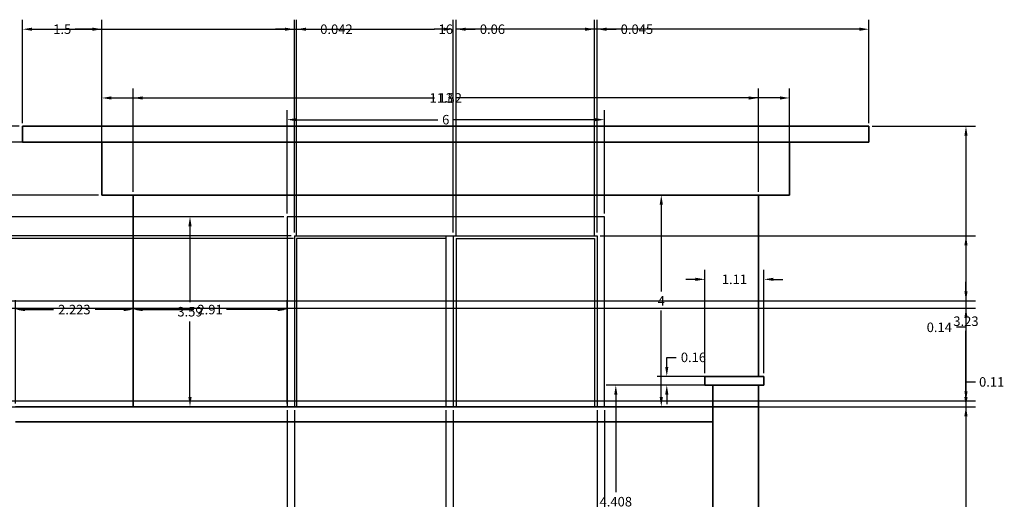
# Model space of a CAD drawing. Units: millimetres. Extents: x 2473 to 2512.3, y 2191.3 to 2230.4.
# Tile 8 of 8: x 2493.7 to 2512.3, y 2221.3 to 2230.4. Entities that reach past the tile are written whole.
import ezdxf

# ---------------------------------------------------------------- set-up
doc = ezdxf.new("R2010")
doc.units = ezdxf.units.MM
for name, color, linetype, lineweight in [('A-ANNO-DIMS', 2, 'Continuous', 18), ('A-ELEV', 7, 'Continuous', 35), ('A-GLAZ', 3, 'Continuous', 25)]:
    doc.layers.add(name, color=color, linetype=linetype, lineweight=lineweight)
doc.styles.get("Standard").update_dxf_attribs({"font": 'arial.ttf'})
doc.dimstyles.get("Standard").update_dxf_attribs({"dimtxt": 0.18, "dimasz": 0.18, "dimexe": 0.18, "dimexo": 0.0625, "dimgap": 0.09, "dimtad": 0, "dimtih": 1, "dimtoh": 1, "dimdec": 4, "dimzin": 0, "dimdsep": 46, "dimtxsty": 'Standard', "dimcen": 0.09, "dimadec": 0, "dimazin": 0, "dimtfac": 1, "dimtdec": 4, "dimtofl": 0, "dimtmove": 0, "dimatfit": 3, "dimfxl": 1, "dimtolj": 1, "dimtzin": 0, "dimarcsym": 0})

# ---------------------------------------------------------------- blocks, each defined once
blk = doc.blocks.new('*D8')
at = {"layer": 'A-ANNO-DIMS', "color": 0, "lineweight": -2, "transparency": 16777216}
for p, q in [((2493.713, 2228.417), (2493.713, 2230.37)), ((2493.893, 2230.19), (2501.503, 2230.19)), ((2509.533, 2230.19), (2501.923, 2230.19)), ((2509.713, 2228.417), (2509.713, 2230.37))]:
    blk.add_line(p, q, dxfattribs=at)
at = {"layer": 'A-ANNO-DIMS', "color": 0, "transparency": 16777216}
for points in [[(2493.893, 2230.22), (2493.893, 2230.16), (2493.713, 2230.19)], [(2509.533, 2230.22), (2509.533, 2230.16), (2509.713, 2230.19)]]:
    blk.add_solid(points, dxfattribs=at)
at = {"layer": 'Defpoints', "color": 0, "transparency": 16777216}
for p in [(2509.713, 2230.19), (2493.713, 2228.355), (2509.713, 2228.355)]:
    blk.add_point(p, dxfattribs=at)
at = {"layer": 'A-ANNO-DIMS', "color": 0, "transparency": 16777216, "insert": (2501.713, 2230.19), "char_height": 0.18, "attachment_point": 5}
blk.add_mtext('\\A1;16', dxfattribs=at)
blk = doc.blocks.new('*D9')
at = {"layer": 'A-ANNO-DIMS', "color": 0, "lineweight": -2, "transparency": 16777216}
for p, q in [((2509.775, 2228.355), (2511.728, 2228.355)), ((2511.548, 2228.175), (2511.548, 2211.037)), ((2511.548, 2193.535), (2511.548, 2210.673)), ((2507.685, 2193.355), (2511.728, 2193.355))]:
    blk.add_line(p, q, dxfattribs=at)
at = {"layer": 'A-ANNO-DIMS', "color": 0, "transparency": 16777216}
for points in [[(2511.518, 2228.175), (2511.578, 2228.175), (2511.548, 2228.355)], [(2511.518, 2193.535), (2511.578, 2193.535), (2511.548, 2193.355)]]:
    blk.add_solid(points, dxfattribs=at)
at = {"layer": 'Defpoints', "color": 0, "transparency": 16777216}
for p in [(2509.713, 2228.355), (2511.548, 2228.355), (2507.623, 2193.355)]:
    blk.add_point(p, dxfattribs=at)
at = {"layer": 'A-ANNO-DIMS', "color": 0, "transparency": 16777216, "insert": (2511.548, 2210.855), "char_height": 0.18, "attachment_point": 5}
blk.add_mtext('\\A1;35', dxfattribs=at)
blk = doc.blocks.new('*D20')
at = {"layer": 'A-ANNO-DIMS', "color": 0, "lineweight": -2, "transparency": 16777216}
for p, q in [((2498.713, 2226.708), (2498.713, 2228.66)), ((2504.713, 2226.708), (2504.713, 2228.66)), ((2498.893, 2228.48), (2501.563, 2228.48)), ((2504.533, 2228.48), (2501.862, 2228.48))]:
    blk.add_line(p, q, dxfattribs=at)
at = {"layer": 'A-ANNO-DIMS', "color": 0, "transparency": 16777216}
for points in [[(2498.893, 2228.51), (2498.893, 2228.45), (2498.713, 2228.48)], [(2504.533, 2228.51), (2504.533, 2228.45), (2504.713, 2228.48)]]:
    blk.add_solid(points, dxfattribs=at)
at = {"layer": 'Defpoints', "color": 0, "transparency": 16777216}
for p in [(2504.713, 2228.48), (2498.713, 2226.645), (2504.713, 2226.645)]:
    blk.add_point(p, dxfattribs=at)
at = {"layer": 'A-ANNO-DIMS', "color": 0, "transparency": 16777216, "insert": (2501.713, 2228.48), "char_height": 0.18, "attachment_point": 5}
blk.add_mtext('\\A1;6', dxfattribs=at)
blk = doc.blocks.new('*D22')
at = {"layer": 'A-ANNO-DIMS', "color": 0, "lineweight": -2, "transparency": 16777216}
for p, q in [((2507.560404, 2227.054888), (2505.607904, 2227.054888)), ((2505.787904, 2226.874888), (2505.787904, 2225.234888)), ((2505.787904, 2223.234888), (2505.787904, 2224.874888)), ((2507.560404, 2223.054888), (2505.607904, 2223.054888))]:
    blk.add_line(p, q, dxfattribs=at)
at = {"layer": 'A-ANNO-DIMS', "color": 0, "transparency": 16777216}
for points in [[(2505.757904, 2226.874888), (2505.817904, 2226.874888), (2505.787904, 2227.054888)], [(2505.757904, 2223.234888), (2505.817904, 2223.234888), (2505.787904, 2223.054888)]]:
    blk.add_solid(points, dxfattribs=at)
at = {"layer": 'Defpoints', "color": 0, "transparency": 16777216}
for p in [(2505.787904, 2227.054888), (2507.622904, 2227.054888), (2507.622904, 2223.054888)]:
    blk.add_point(p, dxfattribs=at)
at = {"layer": 'A-ANNO-DIMS', "color": 0, "transparency": 16777216, "insert": (2505.787904, 2225.054888), "char_height": 0.18, "attachment_point": 5}
blk.add_mtext('\\A1;4', dxfattribs=at)
blk = doc.blocks.new('*D81')
at = {"layer": 'A-ANNO-DIMS', "color": 0, "lineweight": -2, "transparency": 16777216}
for p, q in [((2493.58, 2223.117), (2493.58, 2225.07)), ((2495.803, 2223.117), (2495.803, 2225.07)), ((2493.76, 2224.89), (2494.297, 2224.89)), ((2495.623, 2224.89), (2495.087, 2224.89))]:
    blk.add_line(p, q, dxfattribs=at)
at = {"layer": 'A-ANNO-DIMS', "color": 0, "transparency": 16777216}
for points in [[(2493.76, 2224.92), (2493.76, 2224.86), (2493.58, 2224.89)], [(2495.623, 2224.92), (2495.623, 2224.86), (2495.803, 2224.89)]]:
    blk.add_solid(points, dxfattribs=at)
at = {"layer": 'Defpoints', "color": 0, "transparency": 16777216}
for p in [(2495.803, 2224.89), (2493.58, 2223.055), (2495.803, 2223.055)]:
    blk.add_point(p, dxfattribs=at)
at = {"layer": 'A-ANNO-DIMS', "color": 0, "transparency": 16777216, "insert": (2494.692, 2224.89), "char_height": 0.18, "attachment_point": 5}
blk.add_mtext('\\A1;2.223', dxfattribs=at)
blk = doc.blocks.new('*D82')
at = {"layer": 'A-ANNO-DIMS', "color": 0, "lineweight": -2, "transparency": 16777216}
for p, q in [((2495.803, 2223.117), (2495.803, 2225.07)), ((2498.713, 2223.117), (2498.713, 2225.07)), ((2495.983, 2224.89), (2496.95, 2224.89)), ((2498.533, 2224.89), (2497.566, 2224.89))]:
    blk.add_line(p, q, dxfattribs=at)
at = {"layer": 'A-ANNO-DIMS', "color": 0, "transparency": 16777216}
for points in [[(2495.983, 2224.92), (2495.983, 2224.86), (2495.803, 2224.89)], [(2498.533, 2224.92), (2498.533, 2224.86), (2498.713, 2224.89)]]:
    blk.add_solid(points, dxfattribs=at)
at = {"layer": 'Defpoints', "color": 0, "transparency": 16777216}
for p in [(2498.713, 2224.89), (2495.803, 2223.055), (2498.713, 2223.055)]:
    blk.add_point(p, dxfattribs=at)
at = {"layer": 'A-ANNO-DIMS', "color": 0, "transparency": 16777216, "insert": (2497.258, 2224.89), "char_height": 0.18, "attachment_point": 5}
blk.add_mtext('\\A1;2.91', dxfattribs=at)
blk = doc.blocks.new('*D83')
at = {"layer": 'A-ANNO-DIMS', "color": 0, "lineweight": -2, "transparency": 16777216}
for p, q in [((2495.803, 2227.117), (2495.803, 2229.07)), ((2507.623, 2227.117), (2507.623, 2229.07)), ((2495.983, 2228.89), (2501.329, 2228.89)), ((2507.443, 2228.89), (2502.097, 2228.89))]:
    blk.add_line(p, q, dxfattribs=at)
at = {"layer": 'A-ANNO-DIMS', "color": 0, "transparency": 16777216}
for points in [[(2495.983, 2228.92), (2495.983, 2228.86), (2495.803, 2228.89)], [(2507.443, 2228.92), (2507.443, 2228.86), (2507.623, 2228.89)]]:
    blk.add_solid(points, dxfattribs=at)
at = {"layer": 'Defpoints', "color": 0, "transparency": 16777216}
for p in [(2507.623, 2228.89), (2495.803, 2227.055), (2507.623, 2227.055)]:
    blk.add_point(p, dxfattribs=at)
at = {"layer": 'A-ANNO-DIMS', "color": 0, "transparency": 16777216, "insert": (2501.713, 2228.89), "char_height": 0.18, "attachment_point": 5}
blk.add_mtext('\\A1;11.82', dxfattribs=at)
blk = doc.blocks.new('*D84')
at = {"layer": 'A-ANNO-DIMS', "color": 0, "lineweight": -2, "transparency": 16777216}
for p, q in [((2498.65, 2226.645), (2496.698, 2226.645)), ((2496.878, 2226.465), (2496.878, 2225.032)), ((2496.878, 2223.235), (2496.878, 2224.668)), ((2498.65, 2223.055), (2496.698, 2223.055))]:
    blk.add_line(p, q, dxfattribs=at)
at = {"layer": 'A-ANNO-DIMS', "color": 0, "transparency": 16777216}
for points in [[(2496.848, 2226.465), (2496.908, 2226.465), (2496.878, 2226.645)], [(2496.848, 2223.235), (2496.908, 2223.235), (2496.878, 2223.055)]]:
    blk.add_solid(points, dxfattribs=at)
at = {"layer": 'Defpoints', "color": 0, "transparency": 16777216}
for p in [(2496.878, 2226.645), (2498.713, 2226.645), (2498.713, 2223.055)]:
    blk.add_point(p, dxfattribs=at)
at = {"layer": 'A-ANNO-DIMS', "color": 0, "transparency": 16777216, "insert": (2496.878, 2224.85), "char_height": 0.18, "attachment_point": 5}
blk.add_mtext('\\A1;3.59', dxfattribs=at)
blk = doc.blocks.new('*D85')
at = {"layer": 'A-ANNO-DIMS', "color": 0, "lineweight": -2, "transparency": 16777216}
for p, q in [((2495.15, 2228.055), (2493.198, 2228.055)), ((2493.378, 2227.875), (2493.378, 2227.735)), ((2493.378, 2227.235), (2493.378, 2227.375)), ((2495.15, 2227.055), (2493.198, 2227.055))]:
    blk.add_line(p, q, dxfattribs=at)
at = {"layer": 'A-ANNO-DIMS', "color": 0, "transparency": 16777216}
for points in [[(2493.348, 2227.875), (2493.408, 2227.875), (2493.378, 2228.055)], [(2493.348, 2227.235), (2493.408, 2227.235), (2493.378, 2227.055)]]:
    blk.add_solid(points, dxfattribs=at)
at = {"layer": 'Defpoints', "color": 0, "transparency": 16777216}
for p in [(2493.378, 2228.055), (2495.213, 2228.055), (2495.213, 2227.055)]:
    blk.add_point(p, dxfattribs=at)
at = {"layer": 'A-ANNO-DIMS', "color": 0, "transparency": 16777216, "insert": (2493.378, 2227.555), "char_height": 0.18, "attachment_point": 5}
blk.add_mtext('\\A1;1', dxfattribs=at)
blk = doc.blocks.new('*D86')
at = {"layer": 'A-ANNO-DIMS', "color": 0, "lineweight": -2, "transparency": 16777216}
for p, q in [((2491.878, 2228.535), (2491.878, 2228.715)), ((2491.878, 2228.715), (2492.058, 2228.715)), ((2493.65, 2228.355), (2491.698, 2228.355)), ((2493.65, 2228.055), (2491.698, 2228.055)), ((2491.878, 2227.875), (2491.878, 2227.695))]:
    blk.add_line(p, q, dxfattribs=at)
at = {"layer": 'A-ANNO-DIMS', "color": 0, "transparency": 16777216}
for points in [[(2491.848, 2228.535), (2491.908, 2228.535), (2491.878, 2228.355)], [(2491.848, 2227.875), (2491.908, 2227.875), (2491.878, 2228.055)]]:
    blk.add_solid(points, dxfattribs=at)
at = {"layer": 'Defpoints', "color": 0, "transparency": 16777216}
for p in [(2491.878, 2228.355), (2493.713, 2228.355), (2493.713, 2228.055)]:
    blk.add_point(p, dxfattribs=at)
at = {"layer": 'A-ANNO-DIMS', "color": 0, "transparency": 16777216, "insert": (2492.312, 2228.715), "char_height": 0.18, "attachment_point": 5}
blk.add_mtext('\\A1;0.3', dxfattribs=at)
blk = doc.blocks.new('*D87')
at = {"layer": 'A-ANNO-DIMS', "color": 0, "lineweight": -2, "transparency": 16777216}
for p, q in [((2493.713, 2228.417), (2493.713, 2230.37)), ((2493.893, 2230.19), (2494.217, 2230.19)), ((2495.033, 2230.19), (2494.709, 2230.19)), ((2495.213, 2228.117), (2495.213, 2230.37))]:
    blk.add_line(p, q, dxfattribs=at)
at = {"layer": 'A-ANNO-DIMS', "color": 0, "transparency": 16777216}
for points in [[(2493.893, 2230.22), (2493.893, 2230.16), (2493.713, 2230.19)], [(2495.033, 2230.22), (2495.033, 2230.16), (2495.213, 2230.19)]]:
    blk.add_solid(points, dxfattribs=at)
at = {"layer": 'Defpoints', "color": 0, "transparency": 16777216}
for p in [(2495.213, 2230.19), (2493.713, 2228.355), (2495.213, 2228.055)]:
    blk.add_point(p, dxfattribs=at)
at = {"layer": 'A-ANNO-DIMS', "color": 0, "transparency": 16777216, "insert": (2494.463, 2230.19), "char_height": 0.18, "attachment_point": 5}
blk.add_mtext('\\A1;1.5', dxfattribs=at)
blk = doc.blocks.new('*D88')
at = {"layer": 'A-ANNO-DIMS', "color": 0, "lineweight": -2, "transparency": 16777216}
for p, q in [((2495.213, 2227.117), (2495.213, 2229.07)), ((2508.213, 2227.117), (2508.213, 2229.07)), ((2495.393, 2228.89), (2501.502, 2228.89)), ((2508.033, 2228.89), (2501.923, 2228.89))]:
    blk.add_line(p, q, dxfattribs=at)
at = {"layer": 'A-ANNO-DIMS', "color": 0, "transparency": 16777216}
for points in [[(2495.393, 2228.92), (2495.393, 2228.86), (2495.213, 2228.89)], [(2508.033, 2228.92), (2508.033, 2228.86), (2508.213, 2228.89)]]:
    blk.add_solid(points, dxfattribs=at)
at = {"layer": 'Defpoints', "color": 0, "transparency": 16777216}
for p in [(2508.213, 2228.89), (2495.213, 2227.055), (2508.213, 2227.055)]:
    blk.add_point(p, dxfattribs=at)
at = {"layer": 'A-ANNO-DIMS', "color": 0, "transparency": 16777216, "insert": (2501.713, 2228.89), "char_height": 0.18, "attachment_point": 5}
blk.add_mtext('\\A1;13', dxfattribs=at)
blk = doc.blocks.new('*D90')
at = {"layer": 'A-ANNO-DIMS', "color": 0, "lineweight": -2, "transparency": 16777216}
for p, q in [((2506.614, 2223.689), (2506.614, 2225.642)), ((2507.727, 2223.689), (2507.727, 2225.642)), ((2506.434, 2225.462), (2506.254, 2225.462)), ((2507.907, 2225.462), (2508.087, 2225.462))]:
    blk.add_line(p, q, dxfattribs=at)
at = {"layer": 'A-ANNO-DIMS', "color": 0, "transparency": 16777216}
for points in [[(2506.434, 2225.492), (2506.434, 2225.432), (2506.614, 2225.462)], [(2507.907, 2225.492), (2507.907, 2225.432), (2507.727, 2225.462)]]:
    blk.add_solid(points, dxfattribs=at)
at = {"layer": 'Defpoints', "color": 0, "transparency": 16777216}
for p in [(2507.727, 2225.462), (2506.614, 2223.627), (2507.727, 2223.627)]:
    blk.add_point(p, dxfattribs=at)
at = {"layer": 'A-ANNO-DIMS', "color": 0, "transparency": 16777216, "insert": (2507.171, 2225.462), "char_height": 0.18, "attachment_point": 5}
blk.add_mtext('\\A1;1.11', dxfattribs=at)
blk = doc.blocks.new('*D91')
at = {"layer": 'A-ANNO-DIMS', "color": 0, "lineweight": -2, "transparency": 16777216}
for p, q in [((2506.7, 2223.463), (2504.748, 2223.463)), ((2504.928, 2223.283), (2504.928, 2221.441)), ((2504.928, 2219.235), (2504.928, 2221.077)), ((2506.7, 2219.055), (2504.748, 2219.055))]:
    blk.add_line(p, q, dxfattribs=at)
at = {"layer": 'A-ANNO-DIMS', "color": 0, "transparency": 16777216}
for points in [[(2504.898, 2223.283), (2504.958, 2223.283), (2504.928, 2223.463)], [(2504.898, 2219.235), (2504.958, 2219.235), (2504.928, 2219.055)]]:
    blk.add_solid(points, dxfattribs=at)
at = {"layer": 'Defpoints', "color": 0, "transparency": 16777216}
for p in [(2504.928, 2223.463), (2506.763, 2223.463), (2506.763, 2219.055)]:
    blk.add_point(p, dxfattribs=at)
at = {"layer": 'A-ANNO-DIMS', "color": 0, "transparency": 16777216, "insert": (2504.928, 2221.259), "char_height": 0.18, "attachment_point": 5}
blk.add_mtext('\\A1;4.408', dxfattribs=at)
blk = doc.blocks.new('*D92')
at = {"layer": 'A-ANNO-DIMS', "color": 0, "lineweight": -2, "transparency": 16777216}
for p, q in [((2505.892, 2223.807), (2505.892, 2223.987)), ((2505.892, 2223.987), (2506.072, 2223.987)), ((2507.665, 2223.627), (2505.712, 2223.627)), ((2507.665, 2223.463), (2505.712, 2223.463)), ((2505.892, 2223.283), (2505.892, 2223.103))]:
    blk.add_line(p, q, dxfattribs=at)
at = {"layer": 'A-ANNO-DIMS', "color": 0, "transparency": 16777216}
for points in [[(2505.862, 2223.807), (2505.922, 2223.807), (2505.892, 2223.627)], [(2505.862, 2223.283), (2505.922, 2223.283), (2505.892, 2223.463)]]:
    blk.add_solid(points, dxfattribs=at)
at = {"layer": 'Defpoints', "color": 0, "transparency": 16777216}
for p in [(2505.892, 2223.627), (2507.727, 2223.627), (2507.727, 2223.463)]:
    blk.add_point(p, dxfattribs=at)
at = {"layer": 'A-ANNO-DIMS', "color": 0, "transparency": 16777216, "insert": (2506.396, 2223.987), "char_height": 0.18, "attachment_point": 5}
blk.add_mtext('\\A1;0.16', dxfattribs=at)
blk = doc.blocks.new('*D115')
at = {"layer": 'A-ANNO-DIMS', "color": 0, "lineweight": -2, "transparency": 16777216}
for p, q in [((2498.713, 2222.992), (2498.713, 2191.34)), ((2498.852, 2222.992), (2498.852, 2191.34)), ((2498.533, 2191.52), (2498.353, 2191.52)), ((2499.032, 2191.52), (2499.212, 2191.52))]:
    blk.add_line(p, q, dxfattribs=at)
at = {"layer": 'A-ANNO-DIMS', "color": 0, "transparency": 16777216}
for points in [[(2498.533, 2191.55), (2498.533, 2191.49), (2498.713, 2191.52)], [(2499.032, 2191.55), (2499.032, 2191.49), (2498.852, 2191.52)]]:
    blk.add_solid(points, dxfattribs=at)
at = {"layer": 'Defpoints', "color": 0, "transparency": 16777216}
for p in [(2498.713, 2223.055), (2498.852, 2223.055), (2498.852, 2191.52)]:
    blk.add_point(p, dxfattribs=at)
at = {"layer": 'A-ANNO-DIMS', "color": 0, "transparency": 16777216, "insert": (2499.536, 2191.52), "char_height": 0.18, "attachment_point": 5}
blk.add_mtext('\\A1;0.14', dxfattribs=at)
blk = doc.blocks.new('*D116')
at = {"layer": 'A-ANNO-DIMS', "color": 0, "lineweight": -2, "transparency": 16777216}
for p, q in [((2498.852, 2222.992), (2498.852, 2191.34)), ((2501.713, 2222.992), (2501.713, 2191.34)), ((2499.032, 2191.52), (2499.957, 2191.52)), ((2501.533, 2191.52), (2500.608, 2191.52))]:
    blk.add_line(p, q, dxfattribs=at)
at = {"layer": 'A-ANNO-DIMS', "color": 0, "transparency": 16777216}
for points in [[(2499.032, 2191.55), (2499.032, 2191.49), (2498.852, 2191.52)], [(2501.533, 2191.55), (2501.533, 2191.49), (2501.713, 2191.52)]]:
    blk.add_solid(points, dxfattribs=at)
at = {"layer": 'Defpoints', "color": 0, "transparency": 16777216}
for p in [(2498.852, 2223.055), (2501.713, 2223.055), (2501.713, 2191.52)]:
    blk.add_point(p, dxfattribs=at)
at = {"layer": 'A-ANNO-DIMS', "color": 0, "transparency": 16777216, "insert": (2500.283, 2191.52), "char_height": 0.18, "attachment_point": 5}
blk.add_mtext('\\A1;2.86', dxfattribs=at)
blk = doc.blocks.new('*D117')
at = {"layer": 'A-ANNO-DIMS', "color": 0, "lineweight": -2, "transparency": 16777216}
for p, q in [((2501.713, 2222.992), (2501.713, 2191.34)), ((2501.853, 2222.992), (2501.853, 2191.34)), ((2501.533, 2191.52), (2501.353, 2191.52)), ((2502.033, 2191.52), (2502.213, 2191.52))]:
    blk.add_line(p, q, dxfattribs=at)
at = {"layer": 'A-ANNO-DIMS', "color": 0, "transparency": 16777216}
for points in [[(2501.533, 2191.55), (2501.533, 2191.49), (2501.713, 2191.52)], [(2502.033, 2191.55), (2502.033, 2191.49), (2501.853, 2191.52)]]:
    blk.add_solid(points, dxfattribs=at)
at = {"layer": 'Defpoints', "color": 0, "transparency": 16777216}
for p in [(2501.713, 2223.055), (2501.853, 2223.055), (2501.853, 2191.52)]:
    blk.add_point(p, dxfattribs=at)
at = {"layer": 'A-ANNO-DIMS', "color": 0, "transparency": 16777216, "insert": (2502.536, 2191.52), "char_height": 0.18, "attachment_point": 5}
blk.add_mtext('\\A1;0.14', dxfattribs=at)
blk = doc.blocks.new('*D118')
at = {"layer": 'A-ANNO-DIMS', "color": 0, "lineweight": -2, "transparency": 16777216}
for p, q in [((2501.853, 2222.992), (2501.853, 2191.34)), ((2504.573, 2222.992), (2504.573, 2191.34)), ((2502.033, 2191.52), (2502.888, 2191.52)), ((2504.393, 2191.52), (2503.537, 2191.52))]:
    blk.add_line(p, q, dxfattribs=at)
at = {"layer": 'A-ANNO-DIMS', "color": 0, "transparency": 16777216}
for points in [[(2502.033, 2191.55), (2502.033, 2191.49), (2501.853, 2191.52)], [(2504.393, 2191.55), (2504.393, 2191.49), (2504.573, 2191.52)]]:
    blk.add_solid(points, dxfattribs=at)
at = {"layer": 'Defpoints', "color": 0, "transparency": 16777216}
for p in [(2501.853, 2223.055), (2504.573, 2223.055), (2504.573, 2191.52)]:
    blk.add_point(p, dxfattribs=at)
at = {"layer": 'A-ANNO-DIMS', "color": 0, "transparency": 16777216, "insert": (2503.213, 2191.52), "char_height": 0.18, "attachment_point": 5}
blk.add_mtext('\\A1;2.72', dxfattribs=at)
blk = doc.blocks.new('*D119')
at = {"layer": 'A-ANNO-DIMS', "color": 0, "lineweight": -2, "transparency": 16777216}
for p, q in [((2504.573, 2222.992), (2504.573, 2191.34)), ((2504.713, 2222.992), (2504.713, 2191.34)), ((2504.393, 2191.52), (2504.213, 2191.52)), ((2504.893, 2191.52), (2505.073, 2191.52))]:
    blk.add_line(p, q, dxfattribs=at)
at = {"layer": 'A-ANNO-DIMS', "color": 0, "transparency": 16777216}
for points in [[(2504.393, 2191.55), (2504.393, 2191.49), (2504.573, 2191.52)], [(2504.893, 2191.55), (2504.893, 2191.49), (2504.713, 2191.52)]]:
    blk.add_solid(points, dxfattribs=at)
at = {"layer": 'Defpoints', "color": 0, "transparency": 16777216}
for p in [(2504.573, 2223.055), (2504.713, 2223.055), (2504.713, 2191.52)]:
    blk.add_point(p, dxfattribs=at)
at = {"layer": 'A-ANNO-DIMS', "color": 0, "transparency": 16777216, "insert": (2505.396, 2191.52), "char_height": 0.18, "attachment_point": 5}
blk.add_mtext('\\A1;0.14', dxfattribs=at)
blk = doc.blocks.new('*D120')
at = {"layer": 'A-ANNO-DIMS', "color": 0, "lineweight": -2, "transparency": 16777216}
for p, q in [((2498.672, 2230.19), (2498.492, 2230.19)), ((2498.852, 2226.348), (2498.852, 2230.37)), ((2498.894, 2226.298), (2498.894, 2230.37)), ((2499.074, 2230.19), (2499.254, 2230.19))]:
    blk.add_line(p, q, dxfattribs=at)
at = {"layer": 'A-ANNO-DIMS', "color": 0, "transparency": 16777216}
for points in [[(2498.672, 2230.22), (2498.672, 2230.16), (2498.852, 2230.19)], [(2499.074, 2230.22), (2499.074, 2230.16), (2498.894, 2230.19)]]:
    blk.add_solid(points, dxfattribs=at)
at = {"layer": 'Defpoints', "color": 0, "transparency": 16777216}
for p in [(2498.894, 2230.19), (2498.852, 2226.285), (2498.894, 2226.235)]:
    blk.add_point(p, dxfattribs=at)
at = {"layer": 'A-ANNO-DIMS', "color": 0, "transparency": 16777216, "insert": (2499.647, 2230.19), "char_height": 0.18, "attachment_point": 5}
blk.add_mtext('\\A1;0.042', dxfattribs=at)
blk = doc.blocks.new('*D121')
at = {"layer": 'A-ANNO-DIMS', "color": 0, "lineweight": -2, "transparency": 16777216}
for p, q in [((2501.673, 2230.19), (2501.493, 2230.19)), ((2501.853, 2226.348), (2501.853, 2230.37)), ((2501.912, 2226.298), (2501.912, 2230.37)), ((2502.092, 2230.19), (2502.272, 2230.19))]:
    blk.add_line(p, q, dxfattribs=at)
at = {"layer": 'A-ANNO-DIMS', "color": 0, "transparency": 16777216}
for points in [[(2501.673, 2230.22), (2501.673, 2230.16), (2501.853, 2230.19)], [(2502.092, 2230.22), (2502.092, 2230.16), (2501.912, 2230.19)]]:
    blk.add_solid(points, dxfattribs=at)
at = {"layer": 'Defpoints', "color": 0, "transparency": 16777216}
for p in [(2501.912, 2230.19), (2501.853, 2226.285), (2501.912, 2226.235)]:
    blk.add_point(p, dxfattribs=at)
at = {"layer": 'A-ANNO-DIMS', "color": 0, "transparency": 16777216, "insert": (2502.596, 2230.19), "char_height": 0.18, "attachment_point": 5}
blk.add_mtext('\\A1;0.06', dxfattribs=at)
blk = doc.blocks.new('*D122')
at = {"layer": 'A-ANNO-DIMS', "color": 0, "lineweight": -2, "transparency": 16777216}
for p, q in [((2504.348, 2230.19), (2504.168, 2230.19)), ((2504.528, 2226.298), (2504.528, 2230.37)), ((2504.573, 2226.348), (2504.573, 2230.37)), ((2504.753, 2230.19), (2504.933, 2230.19))]:
    blk.add_line(p, q, dxfattribs=at)
at = {"layer": 'A-ANNO-DIMS', "color": 0, "transparency": 16777216}
for points in [[(2504.348, 2230.22), (2504.348, 2230.16), (2504.528, 2230.19)], [(2504.753, 2230.22), (2504.753, 2230.16), (2504.573, 2230.19)]]:
    blk.add_solid(points, dxfattribs=at)
at = {"layer": 'Defpoints', "color": 0, "transparency": 16777216}
for p in [(2504.573, 2230.19), (2504.573, 2226.285), (2504.528, 2226.235)]:
    blk.add_point(p, dxfattribs=at)
at = {"layer": 'A-ANNO-DIMS', "color": 0, "transparency": 16777216, "insert": (2505.327, 2230.19), "char_height": 0.18, "attachment_point": 5}
blk.add_mtext('\\A1;0.045', dxfattribs=at)
blk = doc.blocks.new('*D123')
at = {"layer": 'A-ANNO-DIMS', "color": 0, "lineweight": -2, "transparency": 16777216}
for p, q in [((2473.788, 2226.825), (2473.788, 2227.005)), ((2498.65, 2226.645), (2473.608, 2226.645)), ((2498.79, 2226.285), (2473.608, 2226.285)), ((2473.788, 2226.105), (2473.788, 2225.925)), ((2473.788, 2225.925), (2473.608, 2225.925))]:
    blk.add_line(p, q, dxfattribs=at)
at = {"layer": 'A-ANNO-DIMS', "color": 0, "transparency": 16777216}
for points in [[(2473.758, 2226.825), (2473.818, 2226.825), (2473.788, 2226.645)], [(2473.758, 2226.105), (2473.818, 2226.105), (2473.788, 2226.285)]]:
    blk.add_solid(points, dxfattribs=at)
at = {"layer": 'Defpoints', "color": 0, "transparency": 16777216}
for p in [(2498.713, 2226.645), (2473.788, 2226.285), (2498.852, 2226.285)]:
    blk.add_point(p, dxfattribs=at)
at = {"layer": 'A-ANNO-DIMS', "color": 0, "transparency": 16777216, "insert": (2473.284, 2225.925), "char_height": 0.18, "attachment_point": 5}
blk.add_mtext('\\A1;0.36', dxfattribs=at)
blk = doc.blocks.new('*D124')
at = {"layer": 'A-ANNO-DIMS', "color": 0, "lineweight": -2, "transparency": 16777216}
for p, q in [((2473.788, 2226.465), (2473.788, 2226.645)), ((2498.79, 2226.285), (2473.608, 2226.285)), ((2498.832, 2226.235), (2473.608, 2226.235)), ((2473.788, 2226.055), (2473.788, 2225.875)), ((2473.788, 2225.875), (2473.608, 2225.875))]:
    blk.add_line(p, q, dxfattribs=at)
at = {"layer": 'A-ANNO-DIMS', "color": 0, "transparency": 16777216}
for points in [[(2473.758, 2226.465), (2473.818, 2226.465), (2473.788, 2226.285)], [(2473.758, 2226.055), (2473.818, 2226.055), (2473.788, 2226.235)]]:
    blk.add_solid(points, dxfattribs=at)
at = {"layer": 'Defpoints', "color": 0, "transparency": 16777216}
for p in [(2498.852, 2226.285), (2473.788, 2226.235), (2498.894, 2226.235)]:
    blk.add_point(p, dxfattribs=at)
at = {"layer": 'A-ANNO-DIMS', "color": 0, "transparency": 16777216, "insert": (2473.283, 2225.875), "char_height": 0.18, "attachment_point": 5}
blk.add_mtext('\\A1;0.05', dxfattribs=at)
blk = doc.blocks.new('*D125')
at = {"layer": 'A-ANNO-DIMS', "color": 0, "lineweight": -2, "transparency": 16777216}
for p, q in [((2504.635, 2226.285), (2511.728, 2226.285)), ((2511.548, 2226.105), (2511.548, 2224.852)), ((2511.548, 2223.235), (2511.548, 2224.488)), ((2504.635, 2223.055), (2511.728, 2223.055))]:
    blk.add_line(p, q, dxfattribs=at)
at = {"layer": 'A-ANNO-DIMS', "color": 0, "transparency": 16777216}
for points in [[(2511.518, 2226.105), (2511.578, 2226.105), (2511.548, 2226.285)], [(2511.518, 2223.235), (2511.578, 2223.235), (2511.548, 2223.055)]]:
    blk.add_solid(points, dxfattribs=at)
at = {"layer": 'Defpoints', "color": 0, "transparency": 16777216}
for p in [(2504.573, 2226.285), (2511.548, 2226.285), (2504.573, 2223.055)]:
    blk.add_point(p, dxfattribs=at)
at = {"layer": 'A-ANNO-DIMS', "color": 0, "transparency": 16777216, "insert": (2511.548, 2224.67), "char_height": 0.18, "attachment_point": 5}
blk.add_mtext('\\A1;3.23', dxfattribs=at)
blk = doc.blocks.new('*D130')
at = {"layer": 'A-ANNO-DIMS', "color": 0, "lineweight": -2, "transparency": 16777216}
for p, q in [((2511.548, 2225.235), (2511.548, 2225.415)), ((2481.978, 2225.055), (2511.728, 2225.055)), ((2481.869, 2224.915), (2511.728, 2224.915)), ((2511.548, 2224.735), (2511.548, 2224.555)), ((2511.548, 2224.555), (2511.368, 2224.555))]:
    blk.add_line(p, q, dxfattribs=at)
at = {"layer": 'A-ANNO-DIMS', "color": 0, "transparency": 16777216}
for points in [[(2511.518, 2225.235), (2511.578, 2225.235), (2511.548, 2225.055)], [(2511.518, 2224.735), (2511.578, 2224.735), (2511.548, 2224.915)]]:
    blk.add_solid(points, dxfattribs=at)
at = {"layer": 'Defpoints', "color": 0, "transparency": 16777216}
for p in [(2481.915, 2225.055), (2481.806, 2224.915), (2511.548, 2224.915)]:
    blk.add_point(p, dxfattribs=at)
at = {"layer": 'A-ANNO-DIMS', "color": 0, "transparency": 16777216, "insert": (2511.044, 2224.555), "char_height": 0.18, "attachment_point": 5}
blk.add_mtext('\\A1;0.14', dxfattribs=at)
blk = doc.blocks.new('*D131')
at = {"layer": 'A-ANNO-DIMS', "color": 0, "lineweight": -2, "transparency": 16777216}
for p, q in [((2511.548, 2223.343), (2511.548, 2223.523)), ((2511.548, 2223.523), (2511.728, 2223.523)), ((2481.869, 2223.163), (2511.728, 2223.163)), ((2481.978, 2223.055), (2511.728, 2223.055)), ((2511.548, 2222.875), (2511.548, 2222.695))]:
    blk.add_line(p, q, dxfattribs=at)
at = {"layer": 'A-ANNO-DIMS', "color": 0, "transparency": 16777216}
for points in [[(2511.518, 2223.343), (2511.578, 2223.343), (2511.548, 2223.163)], [(2511.518, 2222.875), (2511.578, 2222.875), (2511.548, 2223.055)]]:
    blk.add_solid(points, dxfattribs=at)
at = {"layer": 'Defpoints', "color": 0, "transparency": 16777216}
for p in [(2481.806, 2223.163), (2511.548, 2223.163), (2481.915, 2223.055)]:
    blk.add_point(p, dxfattribs=at)
at = {"layer": 'A-ANNO-DIMS', "color": 0, "transparency": 16777216, "insert": (2512.034, 2223.523), "char_height": 0.18, "attachment_point": 5}
blk.add_mtext('\\A1;0.11', dxfattribs=at)

msp = doc.modelspace()

# ---------------------------------------------------------------- linework, layer by layer
at = {"layer": 'A-ELEV'}
for p, q in [((2493.7129, 2228.3549), (2509.7129, 2228.3549)), ((2493.7129, 2228.0549), (2493.7129, 2228.3549)), ((2509.7129, 2228.3549), (2509.7129, 2228.0549)), ((2509.7129, 2228.0549), (2493.7129, 2228.0549)), ((2495.2129, 2227.0549), (2495.2129, 2228.0549)), ((2508.2129, 2228.0549), (2508.2129, 2227.0549)), ((2495.2129, 2227.0549), (2508.2129, 2227.0549)), ((2495.8034, 2227.0549), (2495.8034, 2223.0549)), ((2507.6229, 2227.0549), (2507.6229, 2223.6266)), ((2507.7273, 2223.6266), (2506.6139, 2223.6266)), ((2506.6139, 2223.6266), (2506.6139, 2223.4627)), ((2507.7273, 2223.4627), (2507.7273, 2223.6266)), ((2506.6139, 2223.4627), (2507.7273, 2223.4627)), ((2506.7629, 2219.0549), (2506.7629, 2223.4627)), ((2507.6229, 2223.4627), (2507.6229, 2223.0549)), ((2495.8034, 2223.0549), (2493.5802, 2223.0549)), ((2507.6229, 2223.0549), (2495.8034, 2223.0549)), ((2507.6229, 2223.0549), (2507.6229, 2219.0549)), ((2506.7629, 2222.7699), (2493.5802, 2222.7699))]:
    msp.add_line(p, q, dxfattribs=at)
at = {"layer": 'A-GLAZ'}
for p, q in [((2504.7129, 2226.6451), (2498.7129, 2226.6451)), ((2498.7129, 2226.6451), (2498.7129, 2223.0549)), ((2504.7129, 2223.0549), (2504.7129, 2226.6451)), ((2498.8524, 2226.2854), (2498.8524, 2223.0549)), ((2498.8524, 2226.2854), (2504.5729, 2226.2854)), ((2501.7127, 2226.2854), (2501.7127, 2223.0549)), ((2501.8527, 2226.2854), (2501.8527, 2223.0549)), ((2504.5729, 2226.2854), (2504.5729, 2223.0549)), ((2501.7127, 2226.2352), (2498.8944, 2226.2352)), ((2498.8944, 2226.2352), (2498.8944, 2223.0549)), ((2501.9119, 2226.2352), (2501.9119, 2223.0549)), ((2501.9119, 2226.2352), (2504.528, 2226.2352)), ((2504.528, 2226.2352), (2504.528, 2223.0549))]:
    msp.add_line(p, q, dxfattribs=at)

# ---------------------------------------------------------------- dimensions: what is measured, and where the dimension line sits
at = {"layer": 'A-ANNO-DIMS'}
for base, p1, p2, override, picture, middle in [((2509.7129, 2230.1899), (2493.7129, 2228.3549), (2509.7129, 2228.3549), {"dimdec": 0, "dimlfac": 1, "dimrnd": 0, "dimzin": 0, "dimdsep": 46, "dimlunit": 2}, '*D8', (2501.7129, 2230.1899)), ((2495.2129, 2230.1899), (2493.7129, 2228.3549), (2495.2129, 2228.0549), {"dimdec": 1, "dimlfac": 1, "dimrnd": 0, "dimzin": 0, "dimdsep": 46, "dimlunit": 2}, '*D87', (2494.4629, 2230.1899)), ((2498.8944, 2230.1899), (2498.8524, 2226.2854), (2498.8944, 2226.2352), {"dimdec": 3, "dimlfac": 1, "dimrnd": 0, "dimzin": 0, "dimdsep": 46, "dimlunit": 2}, '*D120', (2499.6472, 2230.1899)), ((2501.9119, 2230.1899), (2501.8527, 2226.2854), (2501.9119, 2226.2352), {"dimdec": 2, "dimlfac": 1, "dimrnd": 0, "dimzin": 0, "dimdsep": 46, "dimlunit": 2}, '*D121', (2502.5956, 2230.1899)), ((2504.5729, 2230.1899), (2504.528, 2226.2352), (2504.5729, 2226.2854), {"dimdec": 3, "dimlfac": 1, "dimrnd": 0, "dimzin": 0, "dimdsep": 46, "dimlunit": 2}, '*D122', (2505.3273, 2230.1899)), ((2508.2129, 2228.8899), (2495.2129, 2227.0549), (2508.2129, 2227.0549), {"dimdec": 0, "dimlfac": 1, "dimrnd": 0, "dimzin": 0, "dimdsep": 46, "dimlunit": 2}, '*D88', (2501.7129, 2228.8899)), ((2507.6229, 2228.8899), (2495.8034, 2227.0549), (2507.6229, 2227.0549), {"dimdec": 2, "dimlfac": 1, "dimrnd": 0, "dimzin": 0, "dimdsep": 46, "dimlunit": 2}, '*D83', (2501.7131, 2228.8899)), ((2504.7129, 2228.4801), (2498.7129, 2226.6451), (2504.7129, 2226.6451), {"dimdec": 0, "dimlfac": 1, "dimrnd": 0, "dimzin": 0, "dimdsep": 46, "dimlunit": 2}, '*D20', (2501.7129, 2228.4801)), ((2507.7273, 2225.4616), (2506.6139, 2223.6266), (2507.7273, 2223.6266), {"dimdec": 2, "dimlfac": 1, "dimrnd": 0, "dimzin": 0, "dimdsep": 46, "dimlunit": 2}, '*D90', (2507.1706, 2225.4616)), ((2495.8034, 2224.8899), (2493.5802, 2223.0549), (2495.8034, 2223.0549), {"dimdec": 3, "dimlfac": 1, "dimrnd": 0, "dimzin": 0, "dimdsep": 46, "dimlunit": 2}, '*D81', (2494.6918, 2224.8899)), ((2498.7129, 2224.8899), (2495.8034, 2223.0549), (2498.7129, 2223.0549), {"dimdec": 2, "dimlfac": 1, "dimrnd": 0, "dimzin": 0, "dimdsep": 46, "dimlunit": 2}, '*D82', (2497.2581, 2224.8899)), ((2498.8524, 2191.5199), (2498.7129, 2223.0549), (2498.8524, 2223.0549), {"dimdec": 2, "dimlfac": 1, "dimrnd": 0, "dimzin": 0, "dimdsep": 46, "dimlunit": 2}, '*D115', (2499.5358, 2191.5199)), ((2501.7127, 2191.5199), (2498.8524, 2223.0549), (2501.7127, 2223.0549), {"dimdec": 2, "dimlfac": 1, "dimrnd": 0, "dimzin": 0, "dimdsep": 46, "dimlunit": 2}, '*D116', (2500.2825, 2191.5199)), ((2501.8527, 2191.5199), (2501.7127, 2223.0549), (2501.8527, 2223.0549), {"dimdec": 2, "dimlfac": 1, "dimrnd": 0, "dimzin": 0, "dimdsep": 46, "dimlunit": 2}, '*D117', (2502.5361, 2191.5199)), ((2504.5729, 2191.5199), (2501.8527, 2223.0549), (2504.5729, 2223.0549), {"dimdec": 2, "dimlfac": 1, "dimrnd": 0, "dimzin": 0, "dimdsep": 46, "dimlunit": 2}, '*D118', (2503.2128, 2191.5199)), ((2504.7129, 2191.5199), (2504.5729, 2223.0549), (2504.7129, 2223.0549), {"dimdec": 2, "dimlfac": 1, "dimrnd": 0, "dimzin": 0, "dimdsep": 46, "dimlunit": 2}, '*D119', (2505.3963, 2191.5199))]:
    dim = msp.add_linear_dim(base=base, p1=p1, p2=p2, dimstyle='Standard', override=override, dxfattribs=at)
    dim.commit()
    dim.dimension.update_dxf_attribs({"geometry": picture, "text_midpoint": middle})
for base, p1, p2, override, picture, middle in [((2491.8779, 2228.3549), (2493.7129, 2228.0549), (2493.7129, 2228.3549), {"dimdec": 1, "dimlfac": 1, "dimrnd": 0, "dimzin": 0, "dimdsep": 46, "dimlunit": 2}, '*D86', (2492.3118, 2228.7149)), ((2511.5479, 2228.3549), (2507.6229, 2193.3549), (2509.7129, 2228.3549), {"dimdec": 0, "dimlfac": 1, "dimrnd": 0, "dimzin": 0, "dimdsep": 46, "dimlunit": 2}, '*D9', (2511.5479, 2210.8549)), ((2493.3779, 2228.0549), (2495.2129, 2227.0549), (2495.2129, 2228.0549), {"dimdec": 0, "dimlfac": 1, "dimrnd": 0, "dimzin": 0, "dimdsep": 46, "dimlunit": 2}, '*D85', (2493.3779, 2227.5549)), ((2505.7879, 2227.0549), (2507.6229, 2223.0549), (2507.6229, 2227.0549), {"dimdec": 0, "dimlfac": 1, "dimrnd": 0, "dimzin": 0, "dimdsep": 46, "dimlunit": 2}, '*D22', (2505.7879, 2225.0549)), ((2473.7879, 2226.2854), (2498.7129, 2226.6451), (2498.8524, 2226.2854), {"dimdec": 2, "dimlfac": 1, "dimrnd": 0, "dimzin": 0, "dimdsep": 46, "dimlunit": 2}, '*D123', (2473.2842, 2225.9254)), ((2473.7879, 2226.2352), (2498.8524, 2226.2854), (2498.8944, 2226.2352), {"dimdec": 2, "dimlfac": 1, "dimrnd": 0, "dimzin": 0, "dimdsep": 46, "dimlunit": 2}, '*D124', (2473.2834, 2225.8752)), ((2496.8779, 2226.6451), (2498.7129, 2223.0549), (2498.7129, 2226.6451), {"dimdec": 2, "dimlfac": 1, "dimrnd": 0, "dimzin": 0, "dimdsep": 46, "dimlunit": 2}, '*D84', (2496.8779, 2224.85)), ((2511.5479, 2226.2854), (2504.5729, 2223.0549), (2504.5729, 2226.2854), {"dimdec": 2, "dimlfac": 1, "dimrnd": 0, "dimzin": 0, "dimdsep": 46, "dimlunit": 2}, '*D125', (2511.5479, 2224.6701)), ((2511.5479, 2224.9147), (2481.9154, 2225.0549), (2481.806, 2224.9147), {"dimdec": 2, "dimlfac": 1, "dimrnd": 0, "dimzin": 0, "dimdsep": 46, "dimlunit": 2}, '*D130', (2511.0445, 2224.5547)), ((2505.8923, 2223.6266), (2507.7273, 2223.4627), (2507.7273, 2223.6266), {"dimdec": 2, "dimlfac": 1, "dimrnd": 0, "dimzin": 0, "dimdsep": 46, "dimlunit": 2}, '*D92', (2506.396, 2223.9866)), ((2511.5479, 2223.1632), (2481.9154, 2223.0549), (2481.806, 2223.1632), {"dimdec": 2, "dimlfac": 1, "dimrnd": 0, "dimzin": 0, "dimdsep": 46, "dimlunit": 2}, '*D131', (2512.0343, 2223.5232)), ((2504.9279, 2223.4627), (2506.7629, 2219.0549), (2506.7629, 2223.4627), {"dimdec": 3, "dimlfac": 1, "dimrnd": 0, "dimzin": 0, "dimdsep": 46, "dimlunit": 2}, '*D91', (2504.9279, 2221.2588))]:
    dim = msp.add_linear_dim(base=base, p1=p1, p2=p2, angle=90, dimstyle='Standard', override=override, dxfattribs=at)
    dim.commit()
    dim.dimension.update_dxf_attribs({"geometry": picture, "text_midpoint": middle})

doc.saveas('drawing.dxf')
